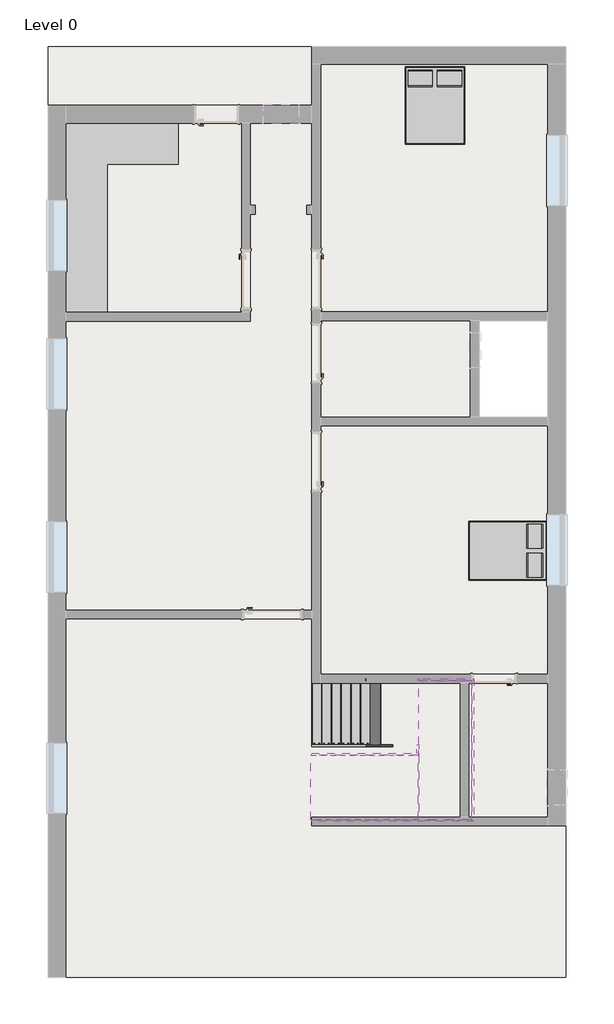
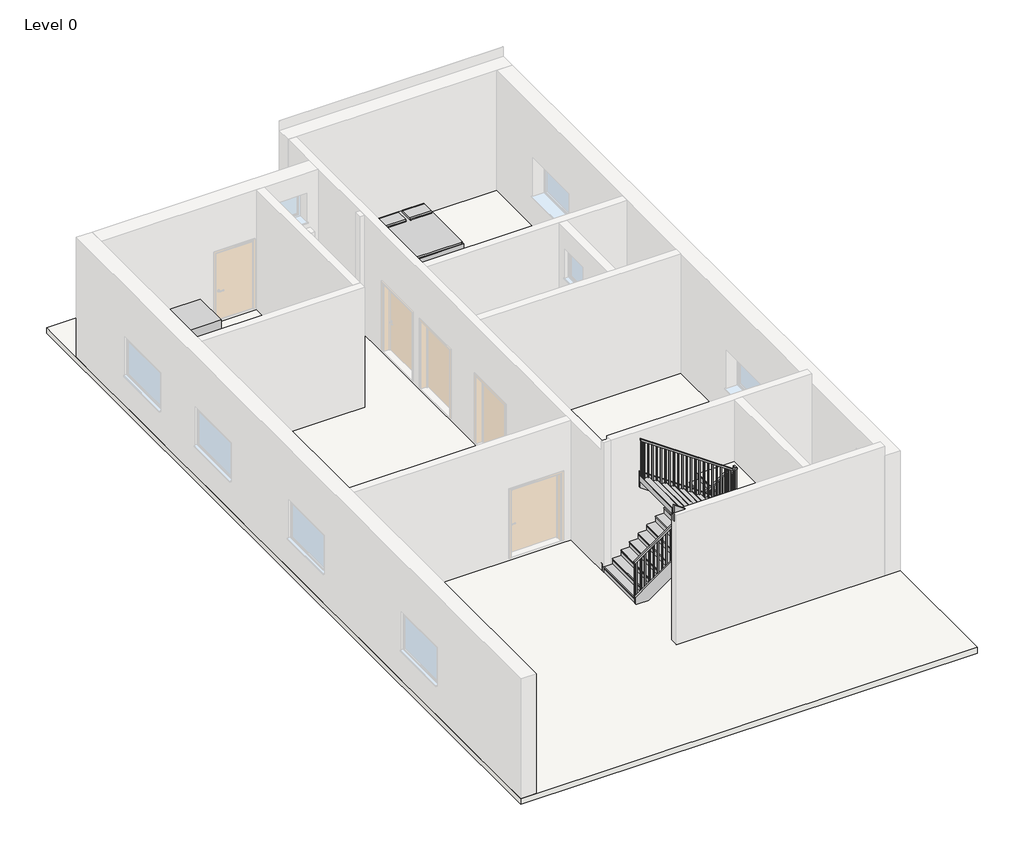
# One storey, part 2 of 2: 8 members, 2 furniture elements, 2 slabs, 2 stair flights, 1 proxy, 1 railing.
"""IFC4 building model written with IfcOpenShell, lengths in millimetres."""

from ifc_helpers import new_model, si_unit, frame, origin, place, context, project, spatial, polyline, outline, extrude, faceted_brep, transform, mapped, element, save
from components import generic_models_1_generic_models_1_540f675e, furniture_bed_1_1525x2007x355mm_queen_b7403446, slab_de2634ce, wood_steps_w_50mm_tread_10mm_nosing_13mm_riser_0f893a5b, wood_steps_w_50mm_tread_10mm_nosing_13mm_riser_e3607291

model = new_model("IFC4")

# Units and contexts
model_context = context("Model", 3, world=origin())
ifc_project = project(units=[si_unit("LENGTHUNIT", "METRE", prefix="MILLI")], contexts=[model_context])

# Site, building, storey
site = spatial("IfcSite", under=ifc_project)
building = spatial("IfcBuilding", under=site)
storey = spatial("IfcBuildingStorey", under=building, Name="Level 0", Elevation=0.0)

# Proxy
placement = place(None, origin())
generic_models_1_generic_models_1_shape = generic_models_1_generic_models_1_540f675e(model_context)
element("IfcBuildingElementProxy", 1, Name="Generic Models 1 : Generic Models 1", ObjectType="Generic Models 1 : Generic Models 1", at=placement, inside=storey, context=model_context, shape_type="MappedRepresentation", body=[
    mapped(generic_models_1_generic_models_1_shape, transform((0.0, 0.0, 0.0), x_axis=(1.0, 0.0, 0.0), y_axis=(0.0, 1.0, 0.0), z_axis=(0.0, 0.0, 1.0))),
])

# Furniture
furniture_bed_1_1525x2007x355mm_queen_shape = furniture_bed_1_1525x2007x355mm_queen_b7403446(model_context)
element("IfcFurniture", 2, ObjectType="Furniture_Bed_1 : 1525x2007x355mm-Queen", at=placement, inside=storey, context=model_context, shape_type="MappedRepresentation", body=[
    mapped(furniture_bed_1_1525x2007x355mm_queen_shape, transform((2305.9986547, 10555.994234, 0.0), x_axis=(1.0, 0.0, 0.0), y_axis=(0.0, 1.0, 0.0), z_axis=(0.0, 0.0, 1.0))),
])
element("IfcFurniture", 3, ObjectType="Furniture_Bed_1 : 1525x2007x355mm-Queen", at=placement, inside=storey, context=model_context, shape_type="MappedRepresentation", body=[
    mapped(furniture_bed_1_1525x2007x355mm_queen_shape, transform((4759.8806219, -806.8828151, 0.0), x_axis=(0.0, -1.0, 0.0), y_axis=(1.0, 0.0, 0.0), z_axis=(0.0, 0.0, 1.0))),
])

# Members
element("IfcMember", 4, ObjectType="Stringer-50mm_Width", at=placement, inside=storey, context=model_context, shape_type="SweptSolid", body=[
    extrude(outline(polyline([(236.4533548, -522.9988863), (0.0, -522.9988863), (0.0, -162.4542975), (1729.3930299, 2323.548183), (2129.3930299, 2198.1018966), (236.4533548, -522.9988863)])), frame((0.0, -4486.6352742, 0.0), z_axis=(0.0, 1.0, 0.0), x_axis=(0.0, 0.0, 1.0)), (0.0, 0.0, 1.0), 50.0),
])
element("IfcMember", 5, ObjectType="Stringer-50mm_Width", at=placement, inside=storey, context=model_context, shape_type="SweptSolid", body=[
    extrude(outline(polyline([(236.4533548, -522.9988863), (0.0, -522.9988863), (0.0, -162.4542975), (1627.4472426, 2177.0011137), (2114.7142244, 2177.0011137), (236.4533548, -522.9988863)])), frame((0.0, -6187.6352742, 0.0), z_axis=(0.0, 1.0, 0.0), x_axis=(0.0, 0.0, 1.0)), (0.0, 0.0, 1.0), 50.0),
])
element("IfcMember", 6, ObjectType="Stringer-50mm_Width", at=placement, inside=storey, context=model_context, shape_type="SweptSolid", body=[
    extrude(outline(polyline([(1729.3930299, 2380.4540445), (2129.3930299, 2505.9003308), (4236.4533548, -522.9988863), (3749.186373, -522.9988863), (1729.3930299, 2380.4540445)])), frame((0.0, -8115.821978, 0.0), z_axis=(0.0, 1.0, 0.0), x_axis=(0.0, 0.0, 1.0)), (0.0, 0.0, 1.0), 50.0),
])
element("IfcMember", 7, ObjectType="Stringer-50mm_Width", at=placement, inside=storey, context=model_context, shape_type="SweptSolid", body=[
    extrude(outline(polyline([(1836.1428948, 2227.0011137), (2323.4098765, 2227.0011137), (4236.4533548, -522.9988863), (3749.186373, -522.9988863), (1836.1428948, 2227.0011137)])), frame((0.0, -6414.821978, 0.0), z_axis=(0.0, 1.0, 0.0), x_axis=(0.0, 0.0, 1.0)), (0.0, 0.0, 1.0), 50.0),
])
element("IfcMember", 8, ObjectType="Stringer-50mm_Width", at=placement, inside=storey, context=model_context, shape_type="Brep", body=[
    faceted_brep([(2505.9003308, -8065.821978, 2129.3930299), (2505.9003308, -8115.821978, 2129.3930299), (3648.1511137, -8115.821978, 2129.3930299), (3598.1511137, -8065.821978, 2129.3930299), (2380.4540445, -8065.821978, 1729.3930299), (3598.1511137, -8065.821978, 1729.3930299), (2380.4540445, -8115.821978, 1729.3930299), (3648.1511137, -8115.821978, 1729.3930299)], [[[0, 1, 2, 3]], [[4, 0, 3, 5]], [[6, 4, 5, 7]], [[1, 6, 7, 2]], [[1, 0, 4, 6]], [[2, 7, 5, 3]]]),
])
element("IfcMember", 9, ObjectType="Stringer-50mm_Width", at=placement, inside=storey, context=model_context, shape_type="SweptSolid", body=[
    extrude(outline(polyline([(3648.1511137, -8115.821978), (3598.1511137, -8065.821978), (3598.1511137, -4486.6352742), (3648.1511137, -4436.6352742), (3648.1511137, -8115.821978)])), frame((0.0, 0.0, 1729.3930299), z_axis=(0.0, 0.0, 1.0), x_axis=(1.0, 0.0, 0.0)), (0.0, 0.0, 1.0), 400.0),
])
element("IfcMember", 10, ObjectType="Stringer-50mm_Width", at=placement, inside=storey, context=model_context, shape_type="Brep", body=[
    faceted_brep([(3598.1511137, -4486.6352742, 2129.3930299), (3648.1511137, -4436.6352742, 2129.3930299), (2198.1018966, -4436.6352742, 2129.3930299), (2198.1018966, -4486.6352742, 2129.3930299), (3598.1511137, -4486.6352742, 1729.3930299), (2323.548183, -4486.6352742, 1729.3930299), (3648.1511137, -4436.6352742, 1729.3930299), (2323.548183, -4436.6352742, 1729.3930299)], [[[0, 1, 2, 3]], [[4, 0, 3, 5]], [[6, 4, 5, 7]], [[1, 6, 7, 2]], [[1, 0, 4, 6]], [[2, 7, 5, 3]]]),
])
element("IfcMember", 11, ObjectType="Stringer-50mm_Width", at=placement, inside=storey, context=model_context, shape_type="SweptSolid", body=[
    extrude(outline(polyline([(2177.0011137, -6137.6352742), (2227.0011137, -6137.6352742), (2227.0011137, -6364.821978), (2177.0011137, -6364.821978), (2177.0011137, -6137.6352742)])), frame((0.0, 0.0, 1729.3930299), z_axis=(0.0, 0.0, 1.0), x_axis=(1.0, 0.0, 0.0)), (0.0, 0.0, 1.0), 400.0),
])

# Railing
element("IfcRailing", 12, ObjectType="1100mm", at=placement, inside=storey, context=model_context, shape_type="SolidModel", body=[
    faceted_brep([(-522.9988863, -6087.2352742, 1273.9130435), (-522.9988863, -6087.2352742, 1213.0046708), (-522.9988863, -6137.2352742, 1213.0046708), (-522.9988863, -6137.2352742, 1273.9130435), (2152.4011137, -6087.2352742, 3135.0608696), (2202.4011137, -6087.2352742, 3108.9351055), (2202.4011137, -6137.2352742, 3108.9351055), (2152.4011137, -6137.2352742, 3135.0608696), (2152.4011137, -6087.2352742, 3186.9565217), (2202.4011137, -6087.2352742, 3136.9565217), (2202.4011137, -6137.2352742, 3136.9565217), (2152.4011137, -6137.2352742, 3186.9565217), (2277.4011137, -6087.2352742, 3186.9565217), (2277.4011137, -6087.2352742, 3136.9565217), (2227.4011137, -6137.2352742, 3136.9565217), (2227.4011137, -6137.2352742, 3186.9565217), (2277.4011137, -6212.2352742, 3186.9565217), (2277.4011137, -6212.2352742, 3136.9565217), (2227.4011137, -6212.2352742, 3136.9565217), (2227.4011137, -6212.2352742, 3186.9565217), (2277.4011137, -6340.221978, 3186.9565217), (2277.4011137, -6390.221978, 3136.9565217), (2227.4011137, -6390.221978, 3136.9565217), (2227.4011137, -6340.221978, 3186.9565217), (2277.4011137, -6340.221978, 3412.7652174), (2277.4011137, -6390.221978, 3362.7652174), (2227.4011137, -6390.221978, 3362.7652174), (2227.4011137, -6340.221978, 3412.7652174), (2277.4011137, -6465.221978, 3412.7652174), (2277.4011137, -6465.221978, 3362.7652174), (2227.4011137, -6415.221978, 3362.7652174), (2227.4011137, -6415.221978, 3412.7652174), (2152.4011137, -6465.221978, 3412.7652174), (2136.7203279, -6465.221978, 3362.7652174), (2136.7203279, -6415.221978, 3362.7652174), (2152.4011137, -6415.221978, 3412.7652174), (-522.9988863, -6465.221978, 5273.9130435), (-522.9988863, -6415.221978, 5273.9130435), (-522.9988863, -6415.221978, 5213.0046708), (-522.9988863, -6465.221978, 5213.0046708)], [[[0, 1, 2, 3]], [[1, 0, 4, 5]], [[2, 1, 5, 6]], [[3, 2, 6, 7]], [[0, 3, 7, 4]], [[5, 4, 8, 9]], [[6, 5, 9, 10]], [[7, 6, 10, 11]], [[4, 7, 11, 8]], [[9, 8, 12, 13]], [[10, 9, 13, 14]], [[11, 10, 14, 15]], [[8, 11, 15, 12]], [[13, 12, 16, 17]], [[14, 13, 17, 18]], [[15, 14, 18, 19]], [[12, 15, 19, 16]], [[17, 16, 20, 21]], [[18, 17, 21, 22]], [[19, 18, 22, 23]], [[16, 19, 23, 20]], [[21, 20, 24, 25]], [[22, 21, 25, 26]], [[23, 22, 26, 27]], [[20, 23, 27, 24]], [[25, 24, 28, 29]], [[26, 25, 29, 30]], [[27, 26, 30, 31]], [[24, 27, 31, 28]], [[29, 28, 32, 33]], [[30, 29, 33, 34]], [[31, 30, 34, 35]], [[28, 31, 35, 32]], [[36, 37, 38, 39]], [[33, 32, 36, 39]], [[34, 33, 39, 38]], [[35, 34, 38, 37]], [[32, 35, 37, 36]]]),
    extrude(outline(polyline([(4000.0, -422.5988863), (5143.1611925, -422.5988863), (5160.5524968, -447.5988863), (4000.0, -447.5988863), (4000.0, -422.5988863)])), frame((0.0, -6452.721978, 0.0), z_axis=(0.0, 1.0, 0.0), x_axis=(0.0, 0.0, 1.0)), (0.0, 0.0, 1.0), 25.0),
    extrude(outline(polyline([(4000.0, -297.5988863), (5056.2046708, -297.5988863), (5073.5959751, -322.5988863), (4000.0, -322.5988863), (4000.0, -297.5988863)])), frame((0.0, -6452.721978, 0.0), z_axis=(0.0, 1.0, 0.0), x_axis=(0.0, 0.0, 1.0)), (0.0, 0.0, 1.0), 25.0),
    extrude(outline(polyline([(3826.0869565, -172.5988863), (4969.248149, -172.5988863), (4986.6394534, -197.5988863), (3826.0869565, -197.5988863), (3826.0869565, -172.5988863)])), frame((0.0, -6452.721978, 0.0), z_axis=(0.0, 1.0, 0.0), x_axis=(0.0, 0.0, 1.0)), (0.0, 0.0, 1.0), 25.0),
    extrude(outline(polyline([(3826.0869565, -47.5988863), (4882.2916273, -47.5988863), (4899.6829316, -72.5988863), (3826.0869565, -72.5988863), (3826.0869565, -47.5988863)])), frame((0.0, -6452.721978, 0.0), z_axis=(0.0, 1.0, 0.0), x_axis=(0.0, 0.0, 1.0)), (0.0, 0.0, 1.0), 25.0),
    extrude(outline(polyline([(3652.173913, 77.4011137), (4795.3351055, 77.4011137), (4812.7264099, 52.4011137), (3652.173913, 52.4011137), (3652.173913, 77.4011137)])), frame((0.0, -6452.721978, 0.0), z_axis=(0.0, 1.0, 0.0), x_axis=(0.0, 0.0, 1.0)), (0.0, 0.0, 1.0), 25.0),
    extrude(outline(polyline([(3652.173913, 202.4011137), (4708.3785838, 202.4011137), (4725.7698881, 177.4011137), (3652.173913, 177.4011137), (3652.173913, 202.4011137)])), frame((0.0, -6452.721978, 0.0), z_axis=(0.0, 1.0, 0.0), x_axis=(0.0, 0.0, 1.0)), (0.0, 0.0, 1.0), 25.0),
    extrude(outline(polyline([(3478.2608696, 327.4011137), (4621.4220621, 327.4011137), (4638.8133664, 302.4011137), (3478.2608696, 302.4011137), (3478.2608696, 327.4011137)])), frame((0.0, -6452.721978, 0.0), z_axis=(0.0, 1.0, 0.0), x_axis=(0.0, 0.0, 1.0)), (0.0, 0.0, 1.0), 25.0),
    extrude(outline(polyline([(3478.2608696, 452.4011137), (4534.4655403, 452.4011137), (4551.8568447, 427.4011137), (3478.2608696, 427.4011137), (3478.2608696, 452.4011137)])), frame((0.0, -6452.721978, 0.0), z_axis=(0.0, 1.0, 0.0), x_axis=(0.0, 0.0, 1.0)), (0.0, 0.0, 1.0), 25.0),
    extrude(outline(polyline([(3304.3478261, 577.4011137), (4447.5090186, 577.4011137), (4464.9003229, 552.4011137), (3304.3478261, 552.4011137), (3304.3478261, 577.4011137)])), frame((0.0, -6452.721978, 0.0), z_axis=(0.0, 1.0, 0.0), x_axis=(0.0, 0.0, 1.0)), (0.0, 0.0, 1.0), 25.0),
    extrude(outline(polyline([(3304.3478261, 702.4011137), (4360.5524968, 702.4011137), (4377.9438012, 677.4011137), (3304.3478261, 677.4011137), (3304.3478261, 702.4011137)])), frame((0.0, -6452.721978, 0.0), z_axis=(0.0, 1.0, 0.0), x_axis=(0.0, 0.0, 1.0)), (0.0, 0.0, 1.0), 25.0),
    extrude(outline(polyline([(3130.4347826, 827.4011137), (4273.5959751, 827.4011137), (4290.9872795, 802.4011137), (3130.4347826, 802.4011137), (3130.4347826, 827.4011137)])), frame((0.0, -6452.721978, 0.0), z_axis=(0.0, 1.0, 0.0), x_axis=(0.0, 0.0, 1.0)), (0.0, 0.0, 1.0), 25.0),
    extrude(outline(polyline([(3130.4347826, 952.4011137), (4186.6394534, 952.4011137), (4204.0307577, 927.4011137), (3130.4347826, 927.4011137), (3130.4347826, 952.4011137)])), frame((0.0, -6452.721978, 0.0), z_axis=(0.0, 1.0, 0.0), x_axis=(0.0, 0.0, 1.0)), (0.0, 0.0, 1.0), 25.0),
    extrude(outline(polyline([(2956.5217391, 1077.4011137), (4099.6829316, 1077.4011137), (4117.074236, 1052.4011137), (2956.5217391, 1052.4011137), (2956.5217391, 1077.4011137)])), frame((0.0, -6452.721978, 0.0), z_axis=(0.0, 1.0, 0.0), x_axis=(0.0, 0.0, 1.0)), (0.0, 0.0, 1.0), 25.0),
    extrude(outline(polyline([(2956.5217391, 1202.4011137), (4012.7264099, 1202.4011137), (4030.1177142, 1177.4011137), (2956.5217391, 1177.4011137), (2956.5217391, 1202.4011137)])), frame((0.0, -6452.721978, 0.0), z_axis=(0.0, 1.0, 0.0), x_axis=(0.0, 0.0, 1.0)), (0.0, 0.0, 1.0), 25.0),
    extrude(outline(polyline([(2782.6086957, 1327.4011137), (3925.7698881, 1327.4011137), (3943.1611925, 1302.4011137), (2782.6086957, 1302.4011137), (2782.6086957, 1327.4011137)])), frame((0.0, -6452.721978, 0.0), z_axis=(0.0, 1.0, 0.0), x_axis=(0.0, 0.0, 1.0)), (0.0, 0.0, 1.0), 25.0),
    extrude(outline(polyline([(2782.6086957, 1452.4011137), (3838.8133664, 1452.4011137), (3856.2046708, 1427.4011137), (2782.6086957, 1427.4011137), (2782.6086957, 1452.4011137)])), frame((0.0, -6452.721978, 0.0), z_axis=(0.0, 1.0, 0.0), x_axis=(0.0, 0.0, 1.0)), (0.0, 0.0, 1.0), 25.0),
    extrude(outline(polyline([(2608.6956522, 1577.4011137), (3751.8568447, 1577.4011137), (3769.248149, 1552.4011137), (2608.6956522, 1552.4011137), (2608.6956522, 1577.4011137)])), frame((0.0, -6452.721978, 0.0), z_axis=(0.0, 1.0, 0.0), x_axis=(0.0, 0.0, 1.0)), (0.0, 0.0, 1.0), 25.0),
    extrude(outline(polyline([(2608.6956522, 1702.4011137), (3664.9003229, 1702.4011137), (3682.2916273, 1677.4011137), (2608.6956522, 1677.4011137), (2608.6956522, 1702.4011137)])), frame((0.0, -6452.721978, 0.0), z_axis=(0.0, 1.0, 0.0), x_axis=(0.0, 0.0, 1.0)), (0.0, 0.0, 1.0), 25.0),
    extrude(outline(polyline([(2434.7826087, 1827.4011137), (3577.9438012, 1827.4011137), (3595.3351055, 1802.4011137), (2434.7826087, 1802.4011137), (2434.7826087, 1827.4011137)])), frame((0.0, -6452.721978, 0.0), z_axis=(0.0, 1.0, 0.0), x_axis=(0.0, 0.0, 1.0)), (0.0, 0.0, 1.0), 25.0),
    extrude(outline(polyline([(2434.7826087, 1952.4011137), (3490.9872795, 1952.4011137), (3508.3785838, 1927.4011137), (2434.7826087, 1927.4011137), (2434.7826087, 1952.4011137)])), frame((0.0, -6452.721978, 0.0), z_axis=(0.0, 1.0, 0.0), x_axis=(0.0, 0.0, 1.0)), (0.0, 0.0, 1.0), 25.0),
    extrude(outline(polyline([(2260.8695652, 2077.4011137), (3404.0307577, 2077.4011137), (3421.4220621, 2052.4011137), (2260.8695652, 2052.4011137), (2260.8695652, 2077.4011137)])), frame((0.0, -6452.721978, 0.0), z_axis=(0.0, 1.0, 0.0), x_axis=(0.0, 0.0, 1.0)), (0.0, 0.0, 1.0), 25.0),
    extrude(outline(polyline([(2202.4011137, -6427.721978), (2202.4011137, -6452.721978), (2177.4011137, -6452.721978), (2177.4011137, -6427.721978), (2202.4011137, -6427.721978)])), frame((0.0, 0.0, 2260.8695652), z_axis=(0.0, 0.0, 1.0), x_axis=(1.0, 0.0, 0.0)), (0.0, 0.0, 1.0), 1101.8956522),
    extrude(outline(polyline([(2239.9011137, -6412.2352742), (2264.9011137, -6412.2352742), (2264.9011137, -6437.2352742), (2239.9011137, -6437.2352742), (2239.9011137, -6412.2352742)])), frame((0.0, 0.0, 2086.9565217), z_axis=(0.0, 0.0, 1.0), x_axis=(1.0, 0.0, 0.0)), (0.0, 0.0, 1.0), 1275.8086957),
    extrude(outline(polyline([(2239.9011137, -6287.2352742), (2264.9011137, -6287.2352742), (2264.9011137, -6312.2352742), (2239.9011137, -6312.2352742), (2239.9011137, -6287.2352742)])), frame((0.0, 0.0, 2086.9565217), z_axis=(0.0, 0.0, 1.0), x_axis=(1.0, 0.0, 0.0)), (0.0, 0.0, 1.0), 1050.0),
    extrude(outline(polyline([(2239.9011137, -6162.2352742), (2264.9011137, -6162.2352742), (2264.9011137, -6187.2352742), (2239.9011137, -6187.2352742), (2239.9011137, -6162.2352742)])), frame((0.0, 0.0, 2086.9565217), z_axis=(0.0, 0.0, 1.0), x_axis=(1.0, 0.0, 0.0)), (0.0, 0.0, 1.0), 1050.0),
    extrude(outline(polyline([(2152.0011137, -6124.7352742), (2152.0011137, -6099.7352742), (2177.0011137, -6099.7352742), (2177.0011137, -6124.7352742), (2152.0011137, -6124.7352742)])), frame((0.0, 0.0, 1913.0434783), z_axis=(0.0, 0.0, 1.0), x_axis=(1.0, 0.0, 0.0)), (0.0, 0.0, 1.0), 1223.9130435),
    extrude(outline(polyline([(2986.9177142, 2027.0011137), (1913.0434783, 2027.0011137), (1913.0434783, 2052.0011137), (3004.3090186, 2052.0011137), (2986.9177142, 2027.0011137)])), frame((0.0, -6124.7352742, 0.0), z_axis=(0.0, 1.0, 0.0), x_axis=(0.0, 0.0, 1.0)), (0.0, 0.0, 1.0), 25.0),
    extrude(outline(polyline([(2899.9611925, 1902.0011137), (1739.1304348, 1902.0011137), (1739.1304348, 1927.0011137), (2917.3524968, 1927.0011137), (2899.9611925, 1902.0011137)])), frame((0.0, -6124.7352742, 0.0), z_axis=(0.0, 1.0, 0.0), x_axis=(0.0, 0.0, 1.0)), (0.0, 0.0, 1.0), 25.0),
    extrude(outline(polyline([(2813.0046708, 1777.0011137), (1739.1304348, 1777.0011137), (1739.1304348, 1802.0011137), (2830.3959751, 1802.0011137), (2813.0046708, 1777.0011137)])), frame((0.0, -6124.7352742, 0.0), z_axis=(0.0, 1.0, 0.0), x_axis=(0.0, 0.0, 1.0)), (0.0, 0.0, 1.0), 25.0),
    extrude(outline(polyline([(2726.048149, 1652.0011137), (1565.2173913, 1652.0011137), (1565.2173913, 1677.0011137), (2743.4394534, 1677.0011137), (2726.048149, 1652.0011137)])), frame((0.0, -6124.7352742, 0.0), z_axis=(0.0, 1.0, 0.0), x_axis=(0.0, 0.0, 1.0)), (0.0, 0.0, 1.0), 25.0),
    extrude(outline(polyline([(2639.0916273, 1527.0011137), (1565.2173913, 1527.0011137), (1565.2173913, 1552.0011137), (2656.4829316, 1552.0011137), (2639.0916273, 1527.0011137)])), frame((0.0, -6124.7352742, 0.0), z_axis=(0.0, 1.0, 0.0), x_axis=(0.0, 0.0, 1.0)), (0.0, 0.0, 1.0), 25.0),
    extrude(outline(polyline([(2552.1351055, 1402.0011137), (1391.3043478, 1402.0011137), (1391.3043478, 1427.0011137), (2569.5264099, 1427.0011137), (2552.1351055, 1402.0011137)])), frame((0.0, -6124.7352742, 0.0), z_axis=(0.0, 1.0, 0.0), x_axis=(0.0, 0.0, 1.0)), (0.0, 0.0, 1.0), 25.0),
    extrude(outline(polyline([(2465.1785838, 1277.0011137), (1391.3043478, 1277.0011137), (1391.3043478, 1302.0011137), (2482.5698881, 1302.0011137), (2465.1785838, 1277.0011137)])), frame((0.0, -6124.7352742, 0.0), z_axis=(0.0, 1.0, 0.0), x_axis=(0.0, 0.0, 1.0)), (0.0, 0.0, 1.0), 25.0),
    extrude(outline(polyline([(2378.2220621, 1152.0011137), (1217.3913043, 1152.0011137), (1217.3913043, 1177.0011137), (2395.6133664, 1177.0011137), (2378.2220621, 1152.0011137)])), frame((0.0, -6124.7352742, 0.0), z_axis=(0.0, 1.0, 0.0), x_axis=(0.0, 0.0, 1.0)), (0.0, 0.0, 1.0), 25.0),
    extrude(outline(polyline([(2291.2655403, 1027.0011137), (1217.3913043, 1027.0011137), (1217.3913043, 1052.0011137), (2308.6568447, 1052.0011137), (2291.2655403, 1027.0011137)])), frame((0.0, -6124.7352742, 0.0), z_axis=(0.0, 1.0, 0.0), x_axis=(0.0, 0.0, 1.0)), (0.0, 0.0, 1.0), 25.0),
    extrude(outline(polyline([(2204.3090186, 902.0011137), (1043.4782609, 902.0011137), (1043.4782609, 927.0011137), (2221.7003229, 927.0011137), (2204.3090186, 902.0011137)])), frame((0.0, -6124.7352742, 0.0), z_axis=(0.0, 1.0, 0.0), x_axis=(0.0, 0.0, 1.0)), (0.0, 0.0, 1.0), 25.0),
    extrude(outline(polyline([(2117.3524968, 777.0011137), (1043.4782609, 777.0011137), (1043.4782609, 802.0011137), (2134.7438012, 802.0011137), (2117.3524968, 777.0011137)])), frame((0.0, -6124.7352742, 0.0), z_axis=(0.0, 1.0, 0.0), x_axis=(0.0, 0.0, 1.0)), (0.0, 0.0, 1.0), 25.0),
    extrude(outline(polyline([(2030.3959751, 652.0011137), (869.5652174, 652.0011137), (869.5652174, 677.0011137), (2047.7872795, 677.0011137), (2030.3959751, 652.0011137)])), frame((0.0, -6124.7352742, 0.0), z_axis=(0.0, 1.0, 0.0), x_axis=(0.0, 0.0, 1.0)), (0.0, 0.0, 1.0), 25.0),
    extrude(outline(polyline([(1943.4394534, 527.0011137), (869.5652174, 527.0011137), (869.5652174, 552.0011137), (1960.8307577, 552.0011137), (1943.4394534, 527.0011137)])), frame((0.0, -6124.7352742, 0.0), z_axis=(0.0, 1.0, 0.0), x_axis=(0.0, 0.0, 1.0)), (0.0, 0.0, 1.0), 25.0),
    extrude(outline(polyline([(1856.4829316, 402.0011137), (695.6521739, 402.0011137), (695.6521739, 427.0011137), (1873.874236, 427.0011137), (1856.4829316, 402.0011137)])), frame((0.0, -6124.7352742, 0.0), z_axis=(0.0, 1.0, 0.0), x_axis=(0.0, 0.0, 1.0)), (0.0, 0.0, 1.0), 25.0),
    extrude(outline(polyline([(1769.5264099, 277.0011137), (695.6521739, 277.0011137), (695.6521739, 302.0011137), (1786.9177142, 302.0011137), (1769.5264099, 277.0011137)])), frame((0.0, -6124.7352742, 0.0), z_axis=(0.0, 1.0, 0.0), x_axis=(0.0, 0.0, 1.0)), (0.0, 0.0, 1.0), 25.0),
    extrude(outline(polyline([(1682.5698881, 152.0011137), (521.7391304, 152.0011137), (521.7391304, 177.0011137), (1699.9611925, 177.0011137), (1682.5698881, 152.0011137)])), frame((0.0, -6124.7352742, 0.0), z_axis=(0.0, 1.0, 0.0), x_axis=(0.0, 0.0, 1.0)), (0.0, 0.0, 1.0), 25.0),
    extrude(outline(polyline([(1595.6133664, 27.0011137), (521.7391304, 27.0011137), (521.7391304, 52.0011137), (1613.0046708, 52.0011137), (1595.6133664, 27.0011137)])), frame((0.0, -6124.7352742, 0.0), z_axis=(0.0, 1.0, 0.0), x_axis=(0.0, 0.0, 1.0)), (0.0, 0.0, 1.0), 25.0),
    extrude(outline(polyline([(1508.6568447, -97.9988863), (347.826087, -97.9988863), (347.826087, -72.9988863), (1526.048149, -72.9988863), (1508.6568447, -97.9988863)])), frame((0.0, -6124.7352742, 0.0), z_axis=(0.0, 1.0, 0.0), x_axis=(0.0, 0.0, 1.0)), (0.0, 0.0, 1.0), 25.0),
    extrude(outline(polyline([(1421.7003229, -222.9988863), (347.826087, -222.9988863), (347.826087, -197.9988863), (1439.0916273, -197.9988863), (1421.7003229, -222.9988863)])), frame((0.0, -6124.7352742, 0.0), z_axis=(0.0, 1.0, 0.0), x_axis=(0.0, 0.0, 1.0)), (0.0, 0.0, 1.0), 25.0),
    extrude(outline(polyline([(1334.7438012, -347.9988863), (173.9130435, -347.9988863), (173.9130435, -322.9988863), (1352.1351055, -322.9988863), (1334.7438012, -347.9988863)])), frame((0.0, -6124.7352742, 0.0), z_axis=(0.0, 1.0, 0.0), x_axis=(0.0, 0.0, 1.0)), (0.0, 0.0, 1.0), 25.0),
    extrude(outline(polyline([(1247.7872795, -472.9988863), (173.9130435, -472.9988863), (173.9130435, -447.9988863), (1265.1785838, -447.9988863), (1247.7872795, -472.9988863)])), frame((0.0, -6124.7352742, 0.0), z_axis=(0.0, 1.0, 0.0), x_axis=(0.0, 0.0, 1.0)), (0.0, 0.0, 1.0), 25.0),
    extrude(outline(polyline([(2239.9011137, -6427.721978), (2264.9011137, -6427.721978), (2264.9011137, -6452.721978), (2239.9011137, -6452.721978), (2239.9011137, -6427.721978)])), frame((0.0, 0.0, 2086.9565217), z_axis=(0.0, 0.0, 1.0), x_axis=(1.0, 0.0, 0.0)), (0.0, 0.0, 1.0), 1275.8086957),
    extrude(outline(polyline([(2239.9011137, -6124.7352742), (2239.9011137, -6099.7352742), (2264.9011137, -6099.7352742), (2264.9011137, -6124.7352742), (2239.9011137, -6124.7352742)])), frame((0.0, 0.0, 2086.9565217), z_axis=(0.0, 0.0, 1.0), x_axis=(1.0, 0.0, 0.0)), (0.0, 0.0, 1.0), 1050.0),
    extrude(outline(polyline([(4000.0, -497.9988863), (5195.6133664, -497.9988863), (5213.0046708, -522.9988863), (4000.0, -522.9988863), (4000.0, -497.9988863)])), frame((0.0, -6452.721978, 0.0), z_axis=(0.0, 1.0, 0.0), x_axis=(0.0, 0.0, 1.0)), (0.0, 0.0, 1.0), 25.0),
    extrude(outline(polyline([(1213.0046708, -522.9988863), (173.9130435, -522.9988863), (173.9130435, -497.9988863), (1230.3959751, -497.9988863), (1213.0046708, -522.9988863)])), frame((0.0, -6124.7352742, 0.0), z_axis=(0.0, 1.0, 0.0), x_axis=(0.0, 0.0, 1.0)), (0.0, 0.0, 1.0), 25.0),
])

# Slabs
slab_shape = slab_de2634ce(model_context)
element("IfcSlab", 13, at=placement, inside=storey, context=model_context, shape_type="MappedRepresentation", body=[
    mapped(slab_shape, transform((0.0, 0.0, 0.0), x_axis=(1.0, 0.0, 0.0), y_axis=(0.0, 1.0, 0.0), z_axis=(0.0, 0.0, 1.0))),
])
element("IfcSlab", 14, ObjectType="Floor-Grnd-Susp_65Scr-80Ins-100Blk-75PC", at=placement, inside=storey, context=model_context, shape_type="SweptSolid", body=[
    extrude(outline(polyline([(6011.1511137, 11833.2891038), (6011.1511137, -4550.1352742), (6011.1511137, -12132.0352742), (-7317.4988863, -12132.0352742), (-7317.4988863, 11833.2891038), (6011.1511137, 11833.2891038)]), holes=[polyline([(5553.9511137, 4777.5566744), (3788.6511137, 4777.5566744), (3788.6511137, 2296.7809218), (5553.9511137, 2296.7809218), (5553.9511137, 4777.5566744)])]), frame((0.0, 0.0, -175.006), z_axis=(0.0, 0.0, 1.0), x_axis=(1.0, 0.0, 0.0)), (0.0, 0.0, 1.0), 175.006),
])

# Stair flights
wood_steps_w_50mm_tread_10mm_nosing_13mm_riser_shape = wood_steps_w_50mm_tread_10mm_nosing_13mm_riser_0f893a5b(model_context)
element("IfcStairFlight", 15, ObjectType="Wood_Steps_w-50mm_Tread-10mm_Nosing-13mm_Riser", at=placement, inside=storey, context=model_context, shape_type="MappedRepresentation", body=[
    mapped(wood_steps_w_50mm_tread_10mm_nosing_13mm_riser_shape, transform((0.0, 0.0, 0.0), x_axis=(1.0, 0.0, 0.0), y_axis=(0.0, 1.0, 0.0), z_axis=(0.0, 0.0, 1.0))),
])
wood_steps_w_50mm_tread_10mm_nosing_13mm_riser_2_shape = wood_steps_w_50mm_tread_10mm_nosing_13mm_riser_e3607291(model_context)
element("IfcStairFlight", 16, ObjectType="Wood_Steps_w-50mm_Tread-10mm_Nosing-13mm_Riser", at=placement, inside=storey, context=model_context, shape_type="MappedRepresentation", body=[
    mapped(wood_steps_w_50mm_tread_10mm_nosing_13mm_riser_2_shape, transform((0.0, 0.0, 0.0), x_axis=(1.0, 0.0, 0.0), y_axis=(0.0, 1.0, 0.0), z_axis=(0.0, 0.0, 1.0))),
])

save(model, "model.ifc")

# Revit data of these elements
# Type "Furniture_Bed_1 : 1525x2007x355mm-Queen"
#   Keynote = "N"
#   Length = 2007 mm
#   Width = 1525 mm
#   Material Frame = Wood - Birch
#   Material Mattress = Textile - White
#   Default Elevation = 0
# Type "1100mm"
#   built-in parameter 1008612 = 0.019685 (stored number, unit not read)
#   built-in parameter 1008611 = 0.019685 (stored number, unit not read)
#   built-in parameter 1008609 = 0.902231 (stored number, unit not read)
#   built-in parameter 1008604 = 0.19685 (stored number, unit not read)
#   built-in parameter 1008603 = 0.164042 (stored number, unit not read)
#   Railing Height = 1100 mm
#   built-in parameter 1008630 = 2
#   built-in parameter 1008610 = 2
#   built-in parameter 1008608 = 1
#   built-in parameter 1008618 = Baluster_Square : 25mm
# Type "Floor-Grnd-Susp_65Scr-80Ins-100Blk-75PC"
#   Keynote = "E60/130"
#   Function = 0
#   Layers, outside or top first: 0 mm "Damp-proofing" (function 100); 100.076 mm "Concrete Masonry, Floor Block" (function 1); 74.93 mm "Concrete, Precast" (function 1)
# Element 1 (IfcBuildingElementProxy, "Generic Models 1 : Generic Models 1")
#   Phase Created = New Construction
# Elements 2, 3 (IfcFurniture, "Furniture_Bed_1 : 1525x2007x355mm-Queen")
#   Phase Created = New Construction
#   Materials on its faces: "Wood - Birch", "Textile - White"
# Elements 4, 5, 6, 7, 8, 9, 10, 11 (IfcMember, "Stringer-50mm_Width")
#   Phase Created = New Construction
# Element 12 (IfcRailing, "1100mm")
#   Phase Created = New Construction
# Element 13 (IfcSlab)
#   Phase Created = New Construction
#   Materials on its faces: "Oak Flooring"
# Element 14 (IfcSlab, "Floor-Grnd-Susp_65Scr-80Ins-100Blk-75PC")
#   Height Offset From Level = 0 mm
#   Phase Created = New Construction
#   Materials on its faces: "Concrete, Precast", "Damp-proofing"
# Elements 15, 16 (IfcStairFlight, "Wood_Steps_w-50mm_Tread-10mm_Nosing-13mm_Riser")
#   Phase Created = New Construction
#   Materials on its faces: "Oak Flooring"
# Materials
#   "Wood - Birch": class "Wood", colour RGB 224 178 126, transparency 0
#   "Textile - White": class "Fabric", colour RGB 247 247 239, transparency 0
#   "Damp-proofing": class "Generic", colour RGB 127 127 127, transparency 0, Description = "Damp-proofing", Cost = 0
#   "Concrete Masonry, Floor Block": class "Concrete", colour RGB 181 181 181, transparency 0, Description = "physical material", Cost = 0
#   "Concrete, Precast": class "Concrete", colour RGB 192 192 192, transparency 0, Description = "Precast concrete", Cost = 0
#   "Oak Flooring": class "Wood", colour RGB 212 179 113, transparency 0, Description = "Quercus Rubra", Cost = 0
